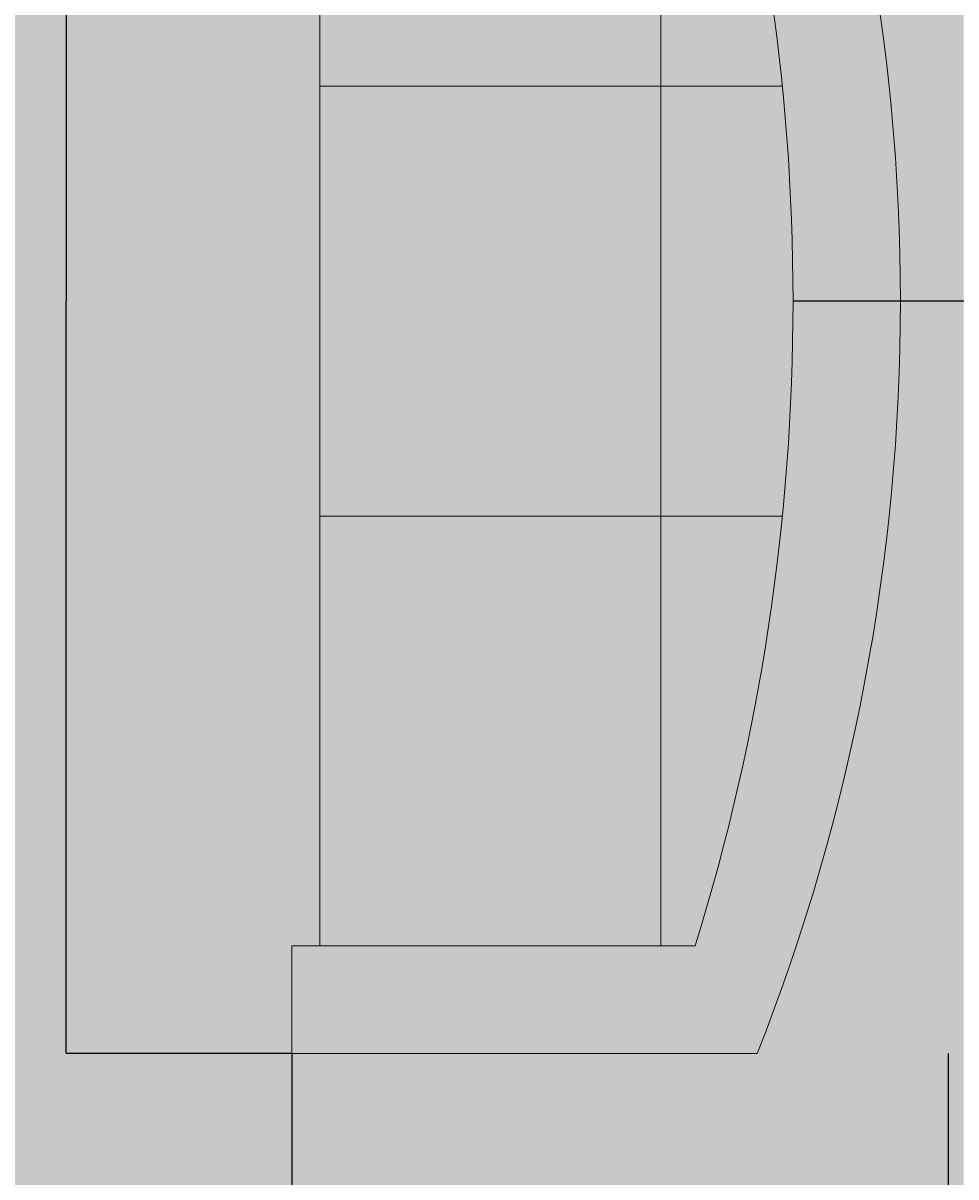
# Model space of a CAD drawing. Units: millimetres. Extents: x -229 to 16545, y -10488 to 4272.
# Tile 18 of 29: x 12629 to 13776, y -4126 to -2708. Entities that reach past the tile are written whole.
import ezdxf

# ---------------------------------------------------------------- set-up
doc = ezdxf.new("R2010")
doc.units = ezdxf.units.MM
for name, color, linetype, lineweight in [('A-ANNO-DIMS', 2, 'Continuous', 18), ('A-FURN', 8, 'Continuous', 18), ('A-FURN-PATT', 252, 'Continuous', 13)]:
    doc.layers.add(name, color=color, linetype=linetype, lineweight=lineweight)
doc.layers.add('A-FLOR-PATT', color=254, linetype='Continuous', lineweight=13, true_color=0xfeeab9)
doc.styles.get("Standard").update_dxf_attribs({"font": 'arial.ttf'})
doc.dimstyles.get("Standard").update_dxf_attribs({"dimtxt": 0.18, "dimasz": 0.18, "dimexe": 0.18, "dimexo": 0.0625, "dimgap": 0.09, "dimtad": 0, "dimtih": 1, "dimtoh": 1, "dimdec": 4, "dimzin": 0, "dimdsep": 46, "dimtxsty": 'Standard', "dimcen": 0.09, "dimadec": 0, "dimazin": 0, "dimtfac": 1, "dimtdec": 4, "dimtofl": 0, "dimtmove": 0, "dimatfit": 3, "dimfxl": 1, "dimtolj": 1, "dimtzin": 0, "dimarcsym": 0})

# ---------------------------------------------------------------- blocks, each defined once
blk = doc.blocks.new('Sofa - Roundback 7 ft.')
for p, q in [((-12.00002, -32.4421), (-12.00003, -6.5971)), ((11.99997, -32.4421), (11.99998, -6.5971)), ((35.99998, -34), (35.99998, -11.4696)), ((-35.999844, -13.3819), (35.9998, -13.3819)), ((-36.000027, -32.4421), (35.99998, -32.4421))]:
    blk.add_line(p, q)
blk.add_lwpolyline([(41.99998, -8), (41.99998, -34), (35.99998, -34)])
for centre, radius, start, end in [((0, -114.25), 114.25, 68.43141, 111.5686), ((-0.00001, -127.1968), 121.1968, 72.72033, 107.2797)]:
    blk.add_arc(centre, radius, start, end)
blk = doc.blocks.new('*D37')
at = {"layer": 'A-ANNO-DIMS', "color": 0, "lineweight": -2, "transparency": 16777216}
for p, q in [((12959.5, -2125.1), (12682, -2125.1)), ((12682.2, -2125.3), (12682.2, -3049.5)), ((12682.2, -3974.1), (12682.2, -3049.9)), ((12959.5, -3974.3), (12682, -3974.3))]:
    blk.add_line(p, q, dxfattribs=at)
at = {"layer": 'A-ANNO-DIMS', "color": 0, "transparency": 16777216}
for points in [[(12682.2, -2125.3), (12682.2, -2125.3), (12682.2, -2125.1)], [(12682.2, -3974.1), (12682.2, -3974.1), (12682.2, -3974.3)]]:
    blk.add_solid(points, dxfattribs=at)
at = {"layer": 'Defpoints', "color": 0, "transparency": 16777216}
for p in [(12959.6, -2125.1), (12682.2, -3974.3), (12959.6, -3974.3)]:
    blk.add_point(p, dxfattribs=at)
at = {"layer": 'A-ANNO-DIMS', "color": 0, "transparency": 16777216, "insert": (12682.2, -3049.7), "char_height": 0.18, "attachment_point": 5}
blk.add_mtext('\\A1;SOFA 1849', dxfattribs=at)
blk = doc.blocks.new('*D38')
at = {"layer": 'A-ANNO-DIMS', "color": 0, "lineweight": -2, "transparency": 16777216}
for p, q in [((12959.6, -3974.4), (12959.6, -4251.9)), ((13766.8, -3974.4), (13766.8, -4251.9)), ((12959.8, -4251.7), (13362.9, -4251.7)), ((13766.6, -4251.7), (13363.5, -4251.7))]:
    blk.add_line(p, q, dxfattribs=at)
at = {"layer": 'A-ANNO-DIMS', "color": 0, "transparency": 16777216}
for points in [[(12959.8, -4251.7), (12959.8, -4251.7), (12959.6, -4251.7)], [(13766.6, -4251.7), (13766.6, -4251.7), (13766.8, -4251.7)]]:
    blk.add_solid(points, dxfattribs=at)
at = {"layer": 'Defpoints', "color": 0, "transparency": 16777216}
for p in [(12959.6, -3974.3), (13766.8, -3974.3), (13766.8, -4251.7)]:
    blk.add_point(p, dxfattribs=at)
at = {"layer": 'A-ANNO-DIMS', "color": 0, "transparency": 16777216, "insert": (13363.2, -4251.7), "char_height": 0.18, "attachment_point": 5}
blk.add_mtext('\\A1;807', dxfattribs=at)
blk = doc.blocks.new('*D101')
at = {"layer": 'A-ANNO-DIMS', "color": 0, "lineweight": -2, "transparency": 16777216}
for p, q in [((10907.8, -3049.7), (10908, -3049.7)), ((10907.9, -3049.8), (10907.9, -3049.6)), ((15176.9, -3049.7), (13576.2, -3049.7))]:
    blk.add_line(p, q, dxfattribs=at)
at = {"layer": 'A-ANNO-DIMS', "color": 0, "transparency": 16777216}
blk.add_solid([(13576.2, -3049.7), (13576.2, -3049.7), (13576, -3049.7)], dxfattribs=at)
at = {"layer": 'Defpoints', "color": 0, "transparency": 16777216}
for p in [(10907.9, -3049.7), (13576, -3049.7)]:
    blk.add_point(p, dxfattribs=at)
at = {"layer": 'A-ANNO-DIMS', "color": 0, "transparency": 16777216, "insert": (15177.3, -3049.7), "char_height": 0.18, "attachment_point": 5}
blk.add_mtext('\\A1;R2668', dxfattribs=at)
blk = doc.blocks.new('*D102')
at = {"layer": 'A-ANNO-DIMS', "color": 0, "lineweight": -2, "transparency": 16777216}
for p, q in [((11192.8, -3049.7), (11193, -3049.7)), ((11192.9, -3049.8), (11192.9, -3049.6)), ((15217.2, -3049.7), (13708.3, -3049.7))]:
    blk.add_line(p, q, dxfattribs=at)
at = {"layer": 'A-ANNO-DIMS', "color": 0, "transparency": 16777216}
blk.add_solid([(13708.3, -3049.7), (13708.3, -3049.7), (13708.1, -3049.7)], dxfattribs=at)
at = {"layer": 'Defpoints', "color": 0, "transparency": 16777216}
for p in [(11192.9, -3049.7), (13708.1, -3049.7)]:
    blk.add_point(p, dxfattribs=at)
at = {"layer": 'A-ANNO-DIMS', "color": 0, "transparency": 16777216, "insert": (15217.6, -3049.7), "char_height": 0.18, "attachment_point": 5}
blk.add_mtext('\\A1;R2515', dxfattribs=at)

msp = doc.modelspace()

# ---------------------------------------------------------------- hatches: boundary and pattern name
at = {"layer": 'A-FLOR-PATT', "transparency": 33554592}
h = msp.add_hatch(color=256, dxfattribs=at)
h.dxf.hatch_style = 1
h.paths.add_polyline_path([(7975.933, -5325.772), (7943.121, -5325.772), (7943.121, -4576.49, 0.40145271), (7225.933, -5325.772, 0.40145271), (6508.746, -4576.49), (6508.746, -5325.772), (6475.933, -5325.772), (6475.933, -5438.272), (5975.933, -5438.272), (5975.933, -7267.724), (5975.933, -7438.272), (6478.619, -7438.272), (6463.448, -7355.919), (6464.88, -7356.837), (6463.849, -7358.097), (6478.619, -7438.272), (6610.327, -7438.272), (6632.656, -7409.564), (6632.525, -7406.967), (6634.208, -7407.569), (6619.273, -7426.77), (6654.466, -7438.272), (7610.517, -7438.272), (7607.41, -7421.409), (7608.842, -7422.327), (7607.812, -7423.587), (7610.517, -7438.272), (7975.933, -7438.272)])
h.paths.add_polyline_path([(13785.933, -1208.272), (9555.933, -1208.272), (9555.933, -961.785), (9705.933, -961.785), (9705.933, -918.035), (10704.976, -918.035, 0.40145271), (9705.933, 38.215), (9555.933, 38.215), (9555.933, 2021.728), (5975.933, 2021.728), (5975.933, 755.492), (5745.933, 755.492), (5745.933, 1427.266), (2918.813, 1427.266), (2918.813, -492.942), (5013.319, -492.942), (5013.319, -978.272), (5745.933, -978.272), (5745.933, -397.513), (5975.933, -397.513), (5975.933, -1208.272), (4560.933, -1208.272), (4560.933, -1265.772), (4448.433, -1265.772), (4448.433, -1298.585), (4445.933, -1298.585), (3699.151, -1298.585, 0.40145271), (4448.433, -2015.772), (4560.933, -2015.772), (4560.933, -2384.177), (5745.933, -2384.177), (5799.402, -2384.177), (5799.402, -4518.272), (5975.933, -4518.272), (5975.933, -5208.272), (6475.933, -5208.272), (6475.933, -4575.772), (6508.746, -4575.772), (6508.746, -4576.49, -0.35647263), (7216.672, -5208.272), (7235.194, -5208.272, -0.35647263), (7943.121, -4576.49), (7943.121, -4575.772), (7975.933, -4575.772), (7975.933, -5208.272), (11176.247, -5208.272), (11159.44, -5191.465), (10520.768, -5191.465), (10520.768, -4888.936), (10571.19, -4888.936), (10571.19, -4872.129), (10772.876, -4872.129), (10772.876, -4888.936), (10789.683, -4888.936), (10789.683, -4872.129), (10991.368, -4872.129), (10991.368, -4888.936), (11041.79, -4888.936), (11041.79, -4872.129), (11058.597, -4872.129, -0.09090909), (11428.354, -4872.129), (11445.162, -4872.129), (11445.162, -4888.936), (11529.197, -4888.936), (11529.197, -5191.465), (11327.512, -5191.465), (11310.704, -5208.272), (13785.933, -5208.272)])
h.paths.add_polyline_path([(11047.216, -1630.944, -1), (11402.816, -1630.944, -1)], flags=16)
h.paths.add_polyline_path([(11148.816, -1630.944), (11225.016, -1554.744), (11301.216, -1630.944), (11225.016, -1707.144)], flags=0)
h.paths.add_polyline_path([(11199.616, -1630.944, -1), (11250.416, -1630.944, -1)], flags=0)
h.paths.add_polyline_path([(11588.751, -2096.259), (11588.751, -1543.254, -0.26666697), (12864.918, -1543.254), (12864.918, -2096.259), (12737.302, -2096.259), (12737.302, -2063.121), (11716.368, -2063.121), (11716.368, -2096.259)], flags=16)
h.paths.add_polyline_path([(12012.696, -2489.42), (12600.997, -2489.42), (12600.997, -3666.022), (12012.696, -3666.022)], flags=16)
h.paths.add_polyline_path([(12176.41, -3599.403), (12174.938, -3609.076), (12173.789, -3618.819), (12173.09, -3628.559), (12172.973, -3638.221), (12173.89, -3652.852), (12175.008, -3657.025), (12172.909, -3643.473), (12173.142, -3624.297), (12175.386, -3605.273)], flags=0)
h.paths.add_polyline_path([(8026.289, -286.944), (7737.703, -287.19), (7734.87, -269.156), (8029.092, -268.905)], flags=16)
h.paths.add_polyline_path([(7733.453, -260.139), (7710.784, -115.865), (7557.191, -115.996), (7556.999, 109.744), (7412.687, 132.166), (7412.433, 429.206), (7556.707, 451.876), (7556.568, 614.769), (7412.256, 637.19), (7412.003, 934.231), (7556.276, 956.9), (7556.084, 1182.639), (7709.677, 1182.77), (7732.099, 1327.082), (8029.14, 1327.335), (8051.808, 1183.062), (8205.401, 1183.192), (8205.594, 957.454), (8349.906, 935.031), (8350.159, 637.99), (8205.885, 615.322), (8206.024, 452.43), (8350.336, 430.006), (8350.59, 132.965), (8206.316, 110.298), (8206.509, -115.442), (8052.916, -115.573), (8030.493, -259.885)], flags=16)
h.paths.add_polyline_path([(12261.416, -3475.554), (12262.632, -3486.776), (12264.032, -3497.007), (12265.554, -3506.365), (12267.136, -3514.968), (12268.719, -3522.935), (12271.304, -3535.59), (12273.606, -3548.078), (12275.271, -3561.064), (12275.93, -3574.938), (12275.325, -3590.3), (12273.425, -3607.964), (12270.795, -3625.658), (12268.066, -3641.063), (12266.318, -3649.679), (12265.456, -3653.626), (12263.984, -3659.846), (12264.032, -3659.566), (12264.342, -3658.241), (12264.807, -3656.37), (12265.456, -3653.626), (12266.318, -3649.679), (12267.409, -3644.302), (12268.668, -3637.664), (12270.019, -3630.037), (12271.384, -3621.695), (12272.69, -3612.908), (12273.857, -3603.948), (12274.81, -3595.088), (12275.47, -3586.601), (12275.782, -3578.689), (12275.757, -3571.292), (12275.423, -3564.275), (12274.816, -3557.512), (12273.964, -3550.872), (12272.896, -3544.224), (12271.645, -3537.439), (12270.24, -3530.385), (12267.543, -3517.181), (12264.612, -3501.247), (12261.849, -3481.059)], flags=0)
h.paths.add_polyline_path([(12332.136, -3408.03), (12333.483, -3416.79), (12335.077, -3424.54), (12336.915, -3431.355), (12338.991, -3437.32), (12341.266, -3442.55), (12343.694, -3447.166), (12346.229, -3451.292), (12348.826, -3455.051), (12351.438, -3458.563), (12357.476, -3466.491), (12363.61, -3476.575), (12368.309, -3489.762), (12369.929, -3503.427), (12369.842, -3516.511), (12368.43, -3530.867), (12365.816, -3545.835), (12362.382, -3559.786), (12360.968, -3564.487), (12363.063, -3557.021), (12364.898, -3549.566), (12366.473, -3542.077), (12367.773, -3534.631), (12368.781, -3527.301), (12369.483, -3520.162), (12369.863, -3513.291), (12369.906, -3506.759), (12369.599, -3500.643), (12368.93, -3494.999), (12367.924, -3489.796), (12366.61, -3484.994), (12365.024, -3480.542), (12363.19, -3476.399), (12361.141, -3472.516), (12358.909, -3468.847), (12356.525, -3465.347), (12354.02, -3461.954), (12351.438, -3458.563), (12345.462, -3450.529), (12339.923, -3439.996), (12335.85, -3428.296), (12332.68, -3412.888)], flags=0)
h.paths.add_polyline_path([(12385.287, -3334.612), (12384.977, -3342.409), (12385.02, -3349.196), (12385.4, -3355.066), (12386.104, -3360.105), (12387.112, -3364.41), (12388.412, -3368.071), (12389.987, -3371.181), (12391.823, -3373.832), (12393.919, -3376.097), (12396.337, -3377.978), (12399.153, -3379.462), (12402.445, -3380.531), (12406.289, -3381.172), (12410.758, -3381.371), (12415.935, -3381.106), (12421.893, -3380.368), (12428.658, -3379.159), (12436.069, -3377.55), (12443.907, -3375.635), (12451.961, -3373.505), (12460.015, -3371.254), (12467.853, -3368.971), (12475.263, -3366.749), (12482.029, -3364.68), (12491.877, -3361.657), (12497.701, -3360.107), (12501.639, -3359.288), (12510.135, -3358.326), (12519.662, -3365.412), (12524.243, -3378.911), (12523.764, -3390.7), (12520.746, -3401.577), (12514.248, -3415.634), (12511.518, -3420.418), (12515.856, -3412.154), (12519.153, -3405.024), (12521.516, -3398.804), (12523.049, -3393.276), (12523.865, -3388.212), (12524.059, -3383.441), (12523.7, -3378.958), (12522.853, -3374.815), (12521.576, -3371.054), (12519.931, -3367.722), (12517.982, -3364.865), (12515.786, -3362.529), (12513.405, -3360.758), (12510.877, -3359.588), (12508.136, -3358.982), (12505.086, -3358.897), (12501.639, -3359.288), (12497.701, -3360.107), (12493.183, -3361.309), (12487.988, -3362.851), (12476.403, -3366.408), (12463.335, -3370.326), (12447.372, -3374.788), (12431.759, -3378.604), (12418.504, -3380.974), (12405.811, -3381.624), (12394.725, -3378.025), (12388.039, -3368.367), (12385.583, -3357.877), (12384.826, -3346.204), (12385.428, -3331.059), (12385.953, -3325.719)], flags=0)
h.paths.add_polyline_path([(7880.016, 1173.969), (7880.373, 1175.495), (7880.433, 1175.851), (7879.484, 1171.818)], flags=0)
h.paths.add_polyline_path([(7802.33, 874.962), (7800.771, 885.032), (7798.932, 893.941), (7796.811, 901.774), (7794.419, 908.63), (7791.798, 914.639), (7789.002, 919.945), (7786.083, 924.686), (7783.093, 929.005), (7780.087, 933.043), (7774.996, 939.717), (7768.406, 949.37), (7762.174, 963.427), (7759.342, 978.002), (7758.629, 991.888), (7759.492, 1007.928), (7761.801, 1025.496), (7765.392, 1044.035), (7766.625, 1049.048), (7764.522, 1039.543), (7762.719, 1030.232), (7761.232, 1021.168), (7760.08, 1012.405), (7759.28, 1003.994), (7758.849, 995.988), (7758.806, 988.44), (7759.167, 981.404), (7759.942, 974.914), (7761.104, 968.936), (7762.617, 963.414), (7764.448, 958.299), (7766.559, 953.535), (7768.918, 949.073), (7771.487, 944.856), (7774.232, 940.835), (7777.115, 936.938), (7782.377, 930.041), (7787.845, 922.139), (7793.348, 911.698), (7798.042, 898.247), (7801.702, 880.527)], flags=0)
h.paths.add_polyline_path([(12519.068, -3228.534), (12519.615, -3236.235), (12520.529, -3242.343), (12521.78, -3247.103), (12523.337, -3250.758), (12525.171, -3253.556), (12527.248, -3255.709), (12529.522, -3257.296), (12531.95, -3258.361), (12534.486, -3258.949), (12537.082, -3259.11), (12539.694, -3258.888), (12542.277, -3258.329), (12544.781, -3257.478), (12547.173, -3256.388), (12549.46, -3255.129), (12550.455, -3254.517), (12555.825, -3251.109), (12557.835, -3249.942), (12565.181, -3246.404), (12574.565, -3253.032), (12576.931, -3265.022), (12576.627, -3277.425), (12575.416, -3290.819), (12574.851, -3295.392), (12575.708, -3287.593), (12576.322, -3280.806), (12576.688, -3274.939), (12576.812, -3269.899), (12576.688, -3265.593), (12576.322, -3261.932), (12575.708, -3258.822), (12574.851, -3256.172), (12573.753, -3253.905), (12572.439, -3252.005), (12570.943, -3250.474), (12569.293, -3249.309), (12567.523, -3248.513), (12565.658, -3248.083), (12563.732, -3248.022), (12561.777, -3248.328), (12559.814, -3248.989), (12557.835, -3249.942), (12555.825, -3251.109), (12553.77, -3252.413), (12551.652, -3253.78), (12549.46, -3255.129), (12543.167, -3258.594), (12532.661, -3259.485), (12524.685, -3253.923), (12520.949, -3245.152), (12519.138, -3233.042)], flags=0)
h.paths.add_polyline_path([(7741.293, 790.501), (7741.641, 799.467), (7741.584, 807.269), (7741.141, 814.015), (7740.329, 819.809), (7739.165, 824.757), (7737.667, 828.966), (7735.853, 832.541), (7733.74, 835.586), (7731.348, 838.188), (7728.71, 840.348), (7725.861, 842.052), (7722.836, 843.28), (7719.671, 844.015), (7716.4, 844.237), (7713.06, 843.932), (7709.684, 843.081), (7706.304, 841.686), (7702.923, 839.834), (7699.543, 837.629), (7696.164, 835.178), (7692.784, 832.585), (7684.718, 826.315), (7675.609, 820.63), (7664.001, 817.274), (7654.105, 821.884), (7647.171, 832.02), (7644.191, 846.522), (7646.321, 860.288), (7647.49, 864.223), (7645.946, 857.865), (7645.046, 852.044), (7644.827, 846.557), (7645.243, 841.404), (7646.221, 836.642), (7647.693, 832.318), (7649.587, 828.489), (7651.832, 825.206), (7654.359, 822.523), (7657.097, 820.49), (7659.984, 819.145), (7662.993, 818.452), (7666.108, 818.357), (7669.311, 818.809), (7672.583, 819.755), (7675.908, 821.139), (7679.268, 822.913), (7682.645, 825.021), (7686.025, 827.401), (7689.404, 829.958), (7692.784, 832.585), (7700.505, 838.509), (7709.871, 843.64), (7721.436, 844.698), (7733.277, 837.617), (7739.571, 825.214), (7741.557, 811.049), (7741.669, 795.575)], flags=0)
h.paths.add_polyline_path([(8377.641, 137.216), (8359.607, 134.382), (8359.356, 428.605), (8377.395, 425.802)], flags=16)
h.paths.add_polyline_path([(7650.715, 668.465), (7650.08, 677.319), (7649.023, 684.34), (7647.579, 689.811), (7645.785, 694.012), (7643.675, 697.228), (7641.286, 699.7), (7638.669, 701.521), (7635.876, 702.744), (7632.96, 703.419), (7629.974, 703.601), (7626.971, 703.344), (7624.004, 702.697), (7621.125, 701.717), (7618.375, 700.462), (7615.749, 699.013), (7614.561, 698.279), (7608.435, 694.382), (7606.125, 693.04), (7598.981, 689.594), (7589.669, 693.773), (7585.26, 702.856), (7584.221, 713.11), (7584.49, 724.584), (7585.863, 739.937), (7586.518, 745.277), (7585.539, 736.31), (7584.841, 728.507), (7584.424, 721.761), (7584.288, 715.966), (7584.433, 711.016), (7584.86, 706.807), (7585.567, 703.231), (7586.556, 700.186), (7587.821, 697.58), (7589.332, 695.397), (7591.053, 693.637), (7592.951, 692.3), (7594.989, 691.385), (7597.132, 690.895), (7599.346, 690.826), (7601.594, 691.18), (7603.851, 691.943), (7606.125, 693.04), (7608.435, 694.382), (7610.797, 695.885), (7613.229, 697.458), (7620.475, 701.929), (7632.001, 704.44), (7643.476, 699.417), (7648.536, 687.571), (7650.63, 673.661)], flags=0)
h.paths.add_polyline_path([(7385.628, 136.37), (7385.382, 424.956), (7403.416, 427.789), (7403.667, 133.567)], flags=16)
h.paths.add_polyline_path([(12993.884, -2257.186), (12959.588, -2257.186), (12959.588, -2125.099), (13531.966, -2125.099, -0.19047621), (13531.966, -3974.321), (12959.588, -3974.321), (12959.588, -3842.233), (12993.884, -3842.233)], flags=16)
h.paths.add_polyline_path([(13413.486, -3313.884), (13413.486, -2785.535), (13562.885, -2785.535, -0.04962821), (13562.885, -3313.884)], flags=0)
h.paths.add_polyline_path([(8377.21, 642.241), (8359.176, 639.407), (8358.925, 933.629), (8376.964, 930.826)], flags=16)
h.paths.add_polyline_path([(13086.058, -1864.83), (13086.058, -1449.84), (13501.048, -1449.84), (13501.048, -1864.83)], flags=16)
h.paths.add_polyline_path([(13305.814, -1862.197), (13302.103, -1859.624), (13298.088, -1857.068), (13293.799, -1854.536), (13289.262, -1852.031), (13284.504, -1849.559), (13279.554, -1847.125), (13274.439, -1844.735), (13269.17, -1842.389), (13263.701, -1840.081), (13257.97, -1837.797), (13251.914, -1835.525), (13245.472, -1833.252), (13238.582, -1830.968), (13231.18, -1828.66), (13223.206, -1826.315), (13209.182, -1822.458), (13204.584, -1821.48), (13217.962, -1824.773), (13235.072, -1829.804), (13248.777, -1834.349), (13260.829, -1838.869), (13274.479, -1844.63), (13289.675, -1852.101), (13302.553, -1859.704)], flags=0)
h.paths.add_polyline_path([(13428.104, -1820.994), (13419.007, -1818.141), (13409.95, -1815.4), (13400.766, -1812.747), (13391.271, -1810.151), (13376.087, -1806.251), (13370.618, -1805.019), (13386.304, -1808.794), (13405.087, -1813.928), (13423.014, -1819.354)], flags=0)
h.paths.add_polyline_path([(7385.197, 641.395), (7384.951, 929.98), (7402.986, 932.814), (7403.236, 638.592)], flags=16)
h.paths.add_polyline_path([(13262.537, -1725.526), (13253.246, -1724.74), (13244.516, -1724.117), (13235.94, -1723.625), (13223.267, -1723.062), (13217.598, -1722.912), (13231.966, -1723.397), (13248.733, -1724.359), (13266.899, -1725.895), (13272.802, -1726.502)], flags=0)
h.paths.add_polyline_path([(13191.893, -1641.137), (13208.675, -1640.506), (13214.057, -1640.258), (13197.763, -1640.936)], flags=0)
h.paths.add_polyline_path([(13097.524, -1608.457), (13114.284, -1609.031), (13120.126, -1609.105), (13103.045, -1608.71)], flags=0)
h.paths.add_polyline_path([(13465.328, -1521.577), (13473.906, -1517.015), (13481.761, -1511.636), (13492.562, -1502.076), (13495.327, -1497.933), (13485.818, -1508.858), (13470.208, -1519.547)], flags=0)
h.paths.add_polyline_path([(13175.015, -1500.891), (13184.046, -1501.807), (13192.721, -1502.52), (13201.114, -1503.034), (13209.273, -1503.351), (13217.244, -1503.476), (13225.078, -1503.41), (13232.821, -1503.16), (13240.524, -1502.728), (13248.233, -1502.117), (13255.993, -1501.322), (13263.825, -1500.293), (13271.746, -1498.974), (13279.775, -1497.305), (13287.928, -1495.229), (13296.222, -1492.688), (13304.675, -1489.622), (13313.304, -1485.975), (13322.089, -1481.727), (13330.859, -1477.028), (13339.408, -1472.063), (13347.526, -1467.02), (13355.006, -1462.087), (13364.86, -1455.202), (13367.224, -1453.299), (13358.544, -1459.754), (13343.348, -1469.775), (13326.143, -1479.767), (13309.023, -1488.045), (13292.249, -1494.129), (13276.009, -1498.264), (13260.299, -1500.88), (13244.401, -1502.51), (13228.945, -1503.378), (13213.316, -1503.508), (13197.047, -1502.876), (13180.088, -1501.481)], flags=0)
h.paths.add_polyline_path([(7733.501, 1336.101), (7736.303, 1354.14), (8024.889, 1354.386), (8027.723, 1336.352)], flags=16)
at = {"layer": 'A-FURN-PATT'}
h = msp.add_hatch(color=256, dxfattribs=at)
h.dxf.hatch_style = 1
h.paths.add_polyline_path([(13413.486, -2257.186), (12993.884, -2257.186), (12993.884, -2785.535), (13413.486, -2785.535)], flags=17)
h.paths.add_polyline_path([(13413.486, -2785.535), (12993.884, -2785.535), (12993.884, -3313.884), (13413.486, -3313.884)], flags=17)
h.paths.add_polyline_path([(13413.486, -3313.884), (12993.884, -3313.884), (12993.884, -3842.233), (13413.486, -3842.233)], flags=17)
h.paths.add_polyline_path([(13531.966, -2125.099), (12959.588, -2125.099), (12959.588, -2257.186), (13455.573, -2257.186, -0.15194781), (13455.573, -3842.233), (12959.588, -3842.233), (12959.588, -3974.321), (13531.966, -3974.321, 0.19047621)])
h.paths.add_polyline_path([(13455.573, -2257.186), (13413.486, -2257.186), (13413.486, -2785.535), (13562.885, -2785.535, 0.05064665)], flags=17)
h.paths.add_polyline_path([(13562.885, -2785.535), (13413.486, -2785.535), (13413.486, -3313.884), (13562.885, -3313.884, 0.04962821)], flags=17)
h.paths.add_polyline_path([(13562.885, -3313.884), (13413.486, -3313.884), (13413.486, -3842.233), (13455.573, -3842.233, 0.05064665)], flags=17)
h.paths.add_polyline_path([(11588.751, -1543.254), (11588.751, -2096.259), (11716.368, -2096.259), (11716.368, -1617.061, -0.22792319), (12737.302, -1617.061), (12737.302, -2096.259), (12864.918, -2096.259), (12864.918, -1543.254, 0.26666697)])
h.paths.add_polyline_path([(12226.834, -1500.713, 0.11251869), (11716.368, -1617.061), (11716.368, -1657.721), (12226.834, -1657.721)], flags=17)
h.paths.add_polyline_path([(12737.302, -1617.061, 0.11251889), (12226.834, -1500.713), (12226.834, -1657.721), (12737.302, -1657.721)], flags=17)
h.paths.add_polyline_path([(12226.834, -1657.721), (11716.368, -1657.721), (11716.368, -2063.121), (12226.834, -2063.121)], flags=17)
h.paths.add_polyline_path([(12737.302, -1657.721), (12226.834, -1657.721), (12226.834, -2063.121), (12737.302, -2063.121)], flags=17)

# ---------------------------------------------------------------- block references
at = {"layer": 'A-FURN', "xscale": 22.01454356165477, "yscale": 22.01454356165477, "zscale": 22.01454356165477, "rotation": 270}
msp.add_blockref('Sofa - Roundback 7 ft.', (13708.082, -3049.71), dxfattribs=at)

# ---------------------------------------------------------------- dimensions: what is measured, and where the dimension line sits
at = {"layer": 'A-ANNO-DIMS'}
dim = msp.add_linear_dim(base=(12682.205, -3974.321), p1=(12959.588, -2125.099), p2=(12959.588, -3974.321), angle=270, text='SOFA <>', dimstyle='Standard', override={"dimdec": 0, "dimlfac": 1, "dimrnd": 0, "dimzin": 0, "dimdsep": 46, "dimlunit": 2}, dxfattribs=at)
dim.commit()
dim.dimension.update_dxf_attribs({"geometry": '*D37', "text_midpoint": (12682.205, -3049.71)})
for center, mpoint, picture, middle in [((10907.903, -3049.71), (13575.995, -3049.709), '*D101', (15176.85, -3049.708)), ((11192.921, -3049.71), (13708.082, -3049.71), '*D102', (15217.179, -3049.71))]:
    dim = msp.add_radius_dim(center=center, mpoint=mpoint, dimstyle='Standard', override={"dimdec": 0, "dimlfac": 1, "dimrnd": 0, "dimzin": 0, "dimdsep": 46, "dimlunit": 2}, dxfattribs=at)
    dim.commit()
    dim.dimension.update_dxf_attribs({"geometry": picture, "text_midpoint": middle, "dimtype": 164})
dim = msp.add_linear_dim(base=(13766.788, -4251.704), p1=(12959.588, -3974.321), p2=(13766.788, -3974.321), dimstyle='Standard', override={"dimdec": 0, "dimlfac": 1, "dimrnd": 0, "dimzin": 0, "dimdsep": 46, "dimlunit": 2}, dxfattribs=at)
dim.commit()
dim.dimension.update_dxf_attribs({"geometry": '*D38', "text_midpoint": (13363.188, -4251.704)})

doc.saveas('drawing.dxf')
